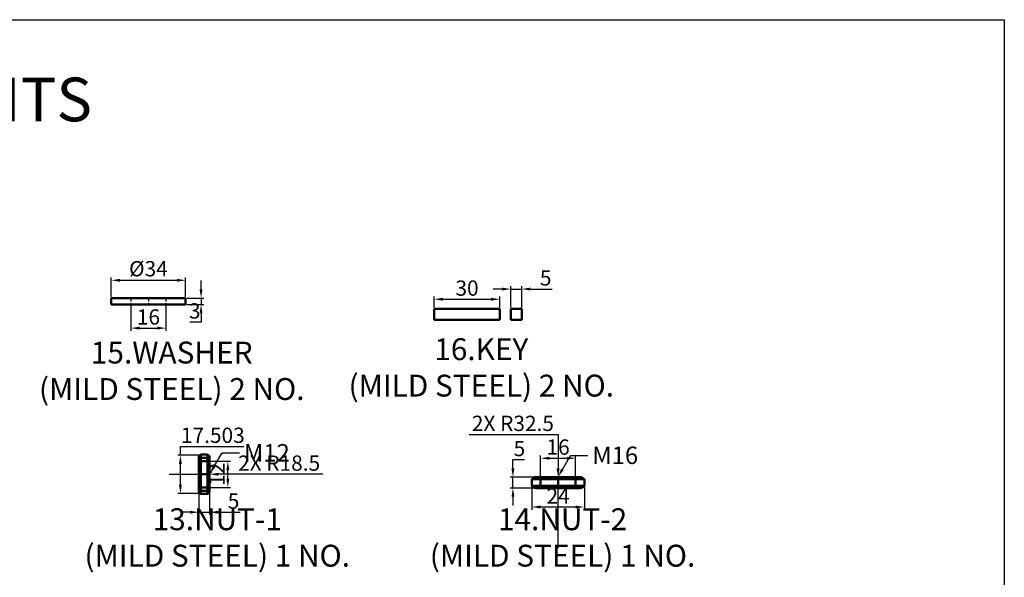
# Model space of a CAD drawing. Units: millimetres. Extents: x -66 to 1195, y -396 to 398.
# Tile 8 of 8: x 745 to 1195, y 143 to 398. Entities that reach past the tile are written whole.
import ezdxf
from ezdxf import colors
from ezdxf.entities.mleader import LeaderData, LeaderLine
from ezdxf.math import Vec2, Vec3

# ---------------------------------------------------------------- set-up
doc = ezdxf.new("R2010")
doc.units = ezdxf.units.MM
doc.header["$LTSCALE"] = 0.5
doc.linetypes.add('HIDDEN', pattern=[9.525, 6.35, -3.175])
for name, color, linetype, lineweight in [('M-DIMS', 2, 'Continuous', 25), ('M-HIDN', 3, 'HIDDEN', 25), ('M-OUTL', 7, 'Continuous', 50), ('M-TEXT', 7, 'Continuous', 25), ('M-TTLB', 7, 'Continuous', 25)]:
    doc.layers.add(name, color=color, linetype=linetype, lineweight=lineweight)
doc.styles.get("Standard").update_dxf_attribs({"font": 'arial.ttf'})
doc.dimstyles.new('ISO-25', dxfattribs={"dimtxt": 7, "dimasz": 4, "dimexe": 1.25, "dimexo": 0.625, "dimtad": 1, "dimtoh": 1, "dimtxsty": 'Standard', "dimcen": 2.5, "dimadec": 0, "dimazin": 0, "dimtfac": 1, "dimtmove": 0, "dimatfit": 3, "dimfxl": 1, "dimarcsym": 0})

# ---------------------------------------------------------------- blocks, each defined once
blk = doc.blocks.new('*D64')
at = {"layer": 'Defpoints', "color": 0, "ltscale": 0.5, "transparency": 16777216}
for p in [(820.76, 278.41), (786.76, 270.29), (820.76, 270.29)]:
    blk.add_point(p, dxfattribs=at)
at = {"layer": 'M-DIMS', "color": 0, "lineweight": -2, "ltscale": 0.5, "transparency": 16777216}
for p, q in [((786.76, 270.91), (786.76, 279.66)), ((820.76, 270.91), (820.76, 279.66)), ((790.76, 278.41), (816.76, 278.41))]:
    blk.add_line(p, q, dxfattribs=at)
at = {"layer": 'M-DIMS', "color": 0, "ltscale": 0.5, "transparency": 16777216}
for points in [[(790.76, 279.08), (790.76, 277.74), (786.76, 278.41)], [(816.76, 279.08), (816.76, 277.74), (820.76, 278.41)]]:
    blk.add_solid(points, dxfattribs=at)
at = {"layer": 'M-DIMS', "color": 0, "ltscale": 0.5, "transparency": 16777216, "insert": (803.76, 282.8), "char_height": 7, "attachment_point": 5}
blk.add_mtext('%%C34', dxfattribs=at)
blk = doc.blocks.new('*D65')
at = {"layer": 'Defpoints', "color": 0, "ltscale": 0.5, "transparency": 16777216}
for p in [(820.76, 270.29), (820.76, 267.29), (827.82, 267.29)]:
    blk.add_point(p, dxfattribs=at)
at = {"layer": 'M-DIMS', "color": 0, "lineweight": -2, "ltscale": 0.5, "transparency": 16777216}
for p, q in [((827.82, 274.29), (827.82, 278.29)), ((821.38, 270.29), (829.07, 270.29)), ((827.82, 270.29), (827.82, 267.29)), ((821.38, 267.29), (829.07, 267.29)), ((827.82, 263.29), (827.82, 259.29)), ((827.82, 259.29), (822.62, 259.29))]:
    blk.add_line(p, q, dxfattribs=at)
at = {"layer": 'M-DIMS', "color": 0, "ltscale": 0.5, "transparency": 16777216}
for points in [[(827.16, 274.29), (828.49, 274.29), (827.82, 270.29)], [(827.16, 263.29), (828.49, 263.29), (827.82, 267.29)]]:
    blk.add_solid(points, dxfattribs=at)
at = {"layer": 'M-DIMS', "color": 0, "ltscale": 0.5, "transparency": 16777216, "insert": (824.91, 263.49), "char_height": 7, "attachment_point": 5}
blk.add_mtext('3', dxfattribs=at)
blk = doc.blocks.new('*D66')
at = {"layer": 'Defpoints', "color": 0, "ltscale": 0.5, "transparency": 16777216}
for p in [(795.76, 267.29), (811.76, 267.29), (811.76, 256.53)]:
    blk.add_point(p, dxfattribs=at)
at = {"layer": 'M-DIMS', "color": 0, "lineweight": -2, "ltscale": 0.5, "transparency": 16777216}
for p, q in [((795.76, 266.66), (795.76, 255.28)), ((811.76, 266.66), (811.76, 255.28)), ((799.76, 256.53), (807.76, 256.53))]:
    blk.add_line(p, q, dxfattribs=at)
at = {"layer": 'M-DIMS', "color": 0, "ltscale": 0.5, "transparency": 16777216}
for points in [[(799.76, 257.2), (799.76, 255.86), (795.76, 256.53)], [(807.76, 257.2), (807.76, 255.86), (811.76, 256.53)]]:
    blk.add_solid(points, dxfattribs=at)
at = {"layer": 'M-DIMS', "color": 0, "ltscale": 0.5, "transparency": 16777216, "insert": (803.76, 260.73), "char_height": 7, "attachment_point": 5}
blk.add_mtext('16', dxfattribs=at)
blk = doc.blocks.new('*D67')
at = {"layer": 'Defpoints', "color": 0, "ltscale": 0.5, "transparency": 16777216}
for p in [(964.42, 269.73), (934.42, 265.35), (964.42, 265.35)]:
    blk.add_point(p, dxfattribs=at)
at = {"layer": 'M-DIMS', "color": 0, "lineweight": -2, "ltscale": 0.5, "transparency": 16777216}
for p, q in [((934.42, 265.97), (934.42, 270.98)), ((964.42, 265.97), (964.42, 270.98)), ((938.42, 269.73), (960.42, 269.73))]:
    blk.add_line(p, q, dxfattribs=at)
at = {"layer": 'M-DIMS', "color": 0, "ltscale": 0.5, "transparency": 16777216}
for points in [[(938.42, 270.4), (938.42, 269.07), (934.42, 269.73)], [(960.42, 270.4), (960.42, 269.07), (964.42, 269.73)]]:
    blk.add_solid(points, dxfattribs=at)
at = {"layer": 'M-DIMS', "color": 0, "ltscale": 0.5, "transparency": 16777216, "insert": (949.42, 273.93), "char_height": 7, "attachment_point": 5}
blk.add_mtext('30', dxfattribs=at)
blk = doc.blocks.new('*D68')
at = {"layer": 'Defpoints', "color": 0, "ltscale": 0.5, "transparency": 16777216}
for p in [(974.42, 274.4), (969.42, 265.35), (974.42, 265.35)]:
    blk.add_point(p, dxfattribs=at)
at = {"layer": 'M-DIMS', "color": 0, "lineweight": -2, "ltscale": 0.5, "transparency": 16777216}
for p, q in [((969.42, 265.97), (969.42, 275.65)), ((974.42, 265.97), (974.42, 275.65)), ((965.42, 274.4), (961.42, 274.4)), ((969.42, 274.4), (974.42, 274.4)), ((978.42, 274.4), (988.31, 274.4))]:
    blk.add_line(p, q, dxfattribs=at)
at = {"layer": 'M-DIMS', "color": 0, "ltscale": 0.5, "transparency": 16777216}
for points in [[(965.42, 275.06), (965.42, 273.73), (969.42, 274.4)], [(978.42, 275.06), (978.42, 273.73), (974.42, 274.4)]]:
    blk.add_solid(points, dxfattribs=at)
at = {"layer": 'M-DIMS', "color": 0, "ltscale": 0.5, "transparency": 16777216, "insert": (985.37, 278.58), "char_height": 7, "attachment_point": 5}
blk.add_mtext('5', dxfattribs=at)
blk = doc.blocks.new('*D109')
at = {"layer": 'Defpoints', "color": 0, "ltscale": 0.5, "transparency": 16777216}
for p in [(818.38, 198.4), (827.32, 198.4), (827.32, 180.9)]:
    blk.add_point(p, dxfattribs=at)
at = {"layer": 'M-DIMS', "color": 0, "lineweight": -2, "ltscale": 0.5, "transparency": 16777216}
for p, q in [((826.7, 198.4), (817.13, 198.4)), ((818.38, 198.4), (818.38, 202.4)), ((818.38, 202.4), (847.41, 202.4)), ((818.38, 184.9), (818.38, 194.4)), ((826.7, 180.9), (817.13, 180.9))]:
    blk.add_line(p, q, dxfattribs=at)
at = {"layer": 'M-DIMS', "color": 0, "ltscale": 0.5, "transparency": 16777216}
for points in [[(817.72, 194.4), (819.05, 194.4), (818.38, 198.4)], [(817.72, 184.9), (819.05, 184.9), (818.38, 180.9)]]:
    blk.add_solid(points, dxfattribs=at)
at = {"layer": 'M-DIMS', "color": 0, "ltscale": 0.5, "transparency": 16777216, "insert": (833.21, 206.6), "char_height": 7, "attachment_point": 5}
blk.add_mtext('17.503', dxfattribs=at)
blk = doc.blocks.new('*D110')
at = {"layer": 'Defpoints', "color": 0, "ltscale": 0.5, "transparency": 16777216}
for p in [(826.73, 189.65), (831.73, 189.65), (831.73, 172.3)]:
    blk.add_point(p, dxfattribs=at)
at = {"layer": 'M-DIMS', "color": 0, "lineweight": -2, "ltscale": 0.5, "transparency": 16777216}
for p, q in [((826.73, 189.02), (826.73, 171.05)), ((831.73, 189.02), (831.73, 171.05)), ((822.73, 172.3), (818.73, 172.3)), ((826.73, 172.3), (831.73, 172.3)), ((835.73, 172.3), (845.63, 172.3))]:
    blk.add_line(p, q, dxfattribs=at)
at = {"layer": 'M-DIMS', "color": 0, "ltscale": 0.5, "transparency": 16777216}
for points in [[(822.73, 172.97), (822.73, 171.63), (826.73, 172.3)], [(835.73, 172.97), (835.73, 171.63), (831.73, 172.3)]]:
    blk.add_solid(points, dxfattribs=at)
at = {"layer": 'M-DIMS', "color": 0, "ltscale": 0.5, "transparency": 16777216, "insert": (842.68, 176.48), "char_height": 7, "attachment_point": 5}
blk.add_mtext('5', dxfattribs=at)
blk = doc.blocks.new('*D111')
at = {"layer": 'Defpoints', "color": 0, "ltscale": 0.5, "transparency": 16777216}
for p in [(831.73, 195.65), (840.08, 195.65), (831.73, 183.65)]:
    blk.add_point(p, dxfattribs=at)
at = {"layer": 'M-DIMS', "color": 0, "lineweight": -2, "ltscale": 0.5, "transparency": 16777216}
for p, q in [((832.36, 195.65), (841.33, 195.65)), ((840.08, 187.65), (840.08, 191.65)), ((832.36, 183.65), (841.33, 183.65))]:
    blk.add_line(p, q, dxfattribs=at)
at = {"layer": 'M-DIMS', "color": 0, "ltscale": 0.5, "transparency": 16777216}
for points in [[(839.42, 191.65), (840.75, 191.65), (840.08, 195.65)], [(839.42, 187.65), (840.75, 187.65), (840.08, 183.65)]]:
    blk.add_solid(points, dxfattribs=at)
at = {"layer": 'M-DIMS', "color": 0, "ltscale": 0.5, "transparency": 16777216, "insert": (835.95, 189.65), "char_height": 7, "attachment_point": 5, "rotation": 90}
blk.add_mtext('12', dxfattribs=at)
blk = doc.blocks.new('*D112')
at = {"layer": 'Defpoints', "color": 0, "ltscale": 0.5, "transparency": 16777216}
for p in [(979.06, 184.34), (1003.06, 184.34), (1003.06, 174.69)]:
    blk.add_point(p, dxfattribs=at)
at = {"layer": 'M-DIMS', "color": 0, "lineweight": -2, "ltscale": 0.5, "transparency": 16777216}
for p, q in [((979.06, 183.72), (979.06, 173.44)), ((1003.06, 183.72), (1003.06, 173.44)), ((983.06, 174.69), (999.06, 174.69))]:
    blk.add_line(p, q, dxfattribs=at)
at = {"layer": 'M-DIMS', "color": 0, "ltscale": 0.5, "transparency": 16777216}
for points in [[(983.06, 175.36), (983.06, 174.02), (979.06, 174.69)], [(999.06, 175.36), (999.06, 174.02), (1003.06, 174.69)]]:
    blk.add_solid(points, dxfattribs=at)
at = {"layer": 'M-DIMS', "color": 0, "ltscale": 0.5, "transparency": 16777216, "insert": (991.06, 178.83), "char_height": 7, "attachment_point": 5}
blk.add_mtext('24', dxfattribs=at)
blk = doc.blocks.new('*D113')
at = {"layer": 'Defpoints', "color": 0, "ltscale": 0.5, "transparency": 16777216}
for p in [(970.41, 188.34), (983.06, 188.34), (983.06, 183.34)]:
    blk.add_point(p, dxfattribs=at)
at = {"layer": 'M-DIMS', "color": 0, "lineweight": -2, "ltscale": 0.5, "transparency": 16777216}
for p, q in [((970.41, 192.34), (970.41, 196.34)), ((970.41, 196.34), (975.68, 196.34)), ((982.44, 188.34), (969.16, 188.34)), ((970.41, 183.34), (970.41, 188.34)), ((982.44, 183.34), (969.16, 183.34)), ((970.41, 179.34), (970.41, 175.34))]:
    blk.add_line(p, q, dxfattribs=at)
at = {"layer": 'M-DIMS', "color": 0, "ltscale": 0.5, "transparency": 16777216}
for points in [[(969.74, 192.34), (971.08, 192.34), (970.41, 188.34)], [(969.74, 179.34), (971.08, 179.34), (970.41, 183.34)]]:
    blk.add_solid(points, dxfattribs=at)
at = {"layer": 'M-DIMS', "color": 0, "ltscale": 0.5, "transparency": 16777216, "insert": (973.36, 200.53), "char_height": 7, "attachment_point": 5}
blk.add_mtext('5', dxfattribs=at)
blk = doc.blocks.new('*D114')
at = {"layer": 'Defpoints', "color": 0, "ltscale": 0.5, "transparency": 16777216}
for p in [(999.06, 197), (983.06, 188.34), (999.06, 188.34)]:
    blk.add_point(p, dxfattribs=at)
at = {"layer": 'M-DIMS', "color": 0, "lineweight": -2, "ltscale": 0.5, "transparency": 16777216}
for p, q in [((983.06, 188.97), (983.06, 198.25)), ((999.06, 188.97), (999.06, 198.25)), ((987.06, 197), (995.06, 197))]:
    blk.add_line(p, q, dxfattribs=at)
at = {"layer": 'M-DIMS', "color": 0, "ltscale": 0.5, "transparency": 16777216}
for points in [[(987.06, 197.66), (987.06, 196.33), (983.06, 197)], [(995.06, 197.66), (995.06, 196.33), (999.06, 197)]]:
    blk.add_solid(points, dxfattribs=at)
at = {"layer": 'M-DIMS', "color": 0, "ltscale": 0.5, "transparency": 16777216, "insert": (991.06, 201.2), "char_height": 7, "attachment_point": 5}
blk.add_mtext('16', dxfattribs=at)
blk = doc.blocks.new('*D133')
at = {"layer": 'Defpoints', "color": 0, "ltscale": 0.5, "transparency": 16777216}
for p in [(813.23, 189.65), (831.73, 189.65)]:
    blk.add_point(p, dxfattribs=at)
at = {"layer": 'M-DIMS', "color": 0, "lineweight": -2, "ltscale": 0.5, "transparency": 16777216}
for p, q in [((813.23, 189.65), (831.73, 189.65)), ((842.83, 189.65), (835.73, 189.65)), ((883.55, 189.65), (842.83, 189.65))]:
    blk.add_line(p, q, dxfattribs=at)
at = {"layer": 'M-DIMS', "color": 0, "ltscale": 0.5, "transparency": 16777216}
blk.add_solid([(835.73, 190.32), (835.73, 188.98), (831.73, 189.65)], dxfattribs=at)
at = {"layer": 'M-DIMS', "color": 0, "ltscale": 0.5, "transparency": 16777216, "insert": (863.51, 193.85), "char_height": 7, "attachment_point": 5}
blk.add_mtext('2X R18.5', dxfattribs=at)
blk = doc.blocks.new('*D134')
at = {"layer": 'Defpoints', "color": 0, "ltscale": 0.5, "transparency": 16777216}
for p in [(991.06, 188.34), (991.06, 155.84)]:
    blk.add_point(p, dxfattribs=at)
at = {"layer": 'M-DIMS', "color": 0, "lineweight": -2, "ltscale": 0.5, "transparency": 16777216}
for p, q in [((950.34, 207.84), (991.06, 207.84)), ((991.06, 207.84), (991.06, 192.34)), ((991.06, 155.84), (991.06, 188.34))]:
    blk.add_line(p, q, dxfattribs=at)
at = {"layer": 'M-DIMS', "color": 0, "ltscale": 0.5, "transparency": 16777216}
blk.add_solid([(991.73, 192.34), (990.39, 192.34), (991.06, 188.34)], dxfattribs=at)
at = {"layer": 'M-DIMS', "color": 0, "ltscale": 0.5, "transparency": 16777216, "insert": (970.39, 212.05), "char_height": 7, "attachment_point": 5}
blk.add_mtext('2X R32.5', dxfattribs=at)

msp = doc.modelspace()

# ---------------------------------------------------------------- linework, layer by layer
at = {"layer": 'M-HIDN', "ltscale": 0.5}
for p, q in [((795.7565, 270.2874), (795.7565, 267.2874)), ((803.7565, 270.2874), (803.7565, 267.2874)), ((811.7565, 270.2874), (811.7565, 267.2874))]:
    msp.add_line(p, q, dxfattribs=at)
at = {"layer": 'M-OUTL', "ltscale": 0.5}
for p, q in [((786.7565, 270.2874), (820.7565, 270.2874)), ((786.7565, 267.2874), (786.7565, 270.2874)), ((820.7565, 270.2874), (820.7565, 267.2874)), ((820.7565, 267.2874), (786.7565, 267.2874)), ((934.4214, 265.3451), (964.4214, 265.3451)), ((934.4214, 260.3451), (934.4214, 265.3451)), ((964.4214, 265.3451), (964.4214, 260.3451)), ((969.4214, 265.3451), (974.4214, 265.3451)), ((969.4214, 260.3451), (969.4214, 265.3451)), ((974.4214, 265.3451), (974.4214, 260.3451)), ((964.4214, 260.3451), (934.4214, 260.3451)), ((974.4214, 260.3451), (969.4214, 260.3451)), ((830.7347, 198.6487), (827.7347, 198.6487)), ((827.7347, 180.6487), (827.7347, 198.6487)), ((830.7347, 180.6487), (830.7347, 198.6487)), ((826.7347, 197.1487), (826.7347, 182.1487)), ((831.7347, 197.1487), (826.7347, 197.1487)), ((826.7347, 182.1487), (826.7347, 197.1487)), ((826.7347, 195.6487), (831.7347, 195.6487)), ((831.7347, 182.1487), (831.7347, 197.1487)), ((826.7347, 189.6487), (831.7347, 189.6487)), ((979.0602, 187.3437), (979.0602, 184.3437)), ((979.0602, 187.3437), (1003.0602, 187.3437)), ((980.9441, 188.3437), (1001.0707, 188.3437)), ((983.0602, 183.3437), (983.0602, 188.3437)), ((991.0602, 188.3437), (991.0602, 183.3437)), ((999.0602, 188.3437), (999.0602, 183.3437)), ((1003.0602, 187.3437), (1003.0602, 184.3437)), ((826.7347, 183.6487), (831.7347, 183.6487)), ((826.7347, 182.1487), (831.7347, 182.1487)), ((827.7347, 180.6487), (830.7347, 180.6487)), ((979.0602, 184.3437), (1003.0602, 184.3437)), ((980.9441, 183.3437), (983.0602, 183.3437)), ((980.9441, 183.3437), (1001.0707, 183.3437)), ((999.0602, 183.3437), (983.0602, 183.3437)), ((1001.0707, 183.3437), (999.0602, 183.3437))]:
    msp.add_line(p, q, dxfattribs=at)
for centre, radius, start, end in [((828.3597, 197.1487), 1.625, 112.619865, 247.380135), ((830.1097, 197.1487), 1.625, 292.619865, 67.380135), ((845.2347, 189.6487), 18.5, 161.075356, 198.924644), ((813.2347, 189.6487), 18.5, 341.075356, 18.924644), ((981.0602, 185.8505), 2.496, 36.745976, 143.254024), ((991.0602, 155.8437), 32.5, 75.749967, 104.250033), ((1001.0602, 185.8438), 2.5, 36.868896, 143.131104), ((828.3597, 182.1487), 1.625, 112.619865, 247.380135), ((830.1097, 182.1487), 1.625, 292.619865, 67.380135), ((981.0602, 185.837), 2.496, 216.745976, 323.254024), ((991.0602, 215.8437), 32.5, 255.749967, 284.250033), ((1001.0602, 185.8437), 2.5, 216.868896, 323.131104)]:
    msp.add_arc(centre, radius, start, end, dxfattribs=at)
at = {"layer": 'M-TTLB', "ltscale": 0.5}
msp.add_lwpolyline([(-66.4176, 397.641), (1195.0519, 397.641), (1195.0519, -395.6964), (-66.4176, -395.6964)], close=True, dxfattribs=at)

# ---------------------------------------------------------------- texts
at = {"layer": 'M-TEXT', "ltscale": 0.5, "attachment_point": 1}
for s, width, insert, char_height in [('LATHE TAIL STOCK COMPONENTS ', 485.790741, (346.8576, 371.1482), 20), ('\\pxqc;15.WASHER \\P(MILD STEEL) 2 NO.', 203.992441, (712.4274, 250.3326), 10), ('\\pxqc;16.KEY \\P(MILD STEEL) 2 NO.', 203.992441, (853.9471, 251.883), 10), ('\\pxqc;13.NUT-1\\P(MILD STEEL) 1 NO.', 203.992441, (733.2302, 174.0776), 10), ('\\pxqc;14.NUT-2\\P(MILD STEEL) 1 NO.', 203.992441, (891.0952, 174.0776), 10)]:
    msp.add_mtext_dynamic_manual_height_columns(s, width=width, gutter_width=12.5, heights=[0], dxfattribs=dict(at, insert=insert, char_height=char_height))

# ---------------------------------------------------------------- dimensions: what is measured, and where the dimension line sits
at = {"layer": 'M-DIMS', "ltscale": 0.5}
dim = msp.add_linear_dim(base=(820.7565, 278.4092), p1=(786.7565, 270.2874), p2=(820.7565, 270.2874), text='%%C<>', dimstyle='ISO-25', override={"dimclrd": 0, "dimclre": 0, "dimclrt": 0}, dxfattribs=at)
dim.commit()
dim.dimension.update_dxf_attribs({"geometry": '*D64', "text_midpoint": (803.7565, 282.8039)})
for base, p1, p2, override, picture, middle in [((974.4214, 274.3973), (969.4214, 265.3451), (974.4214, 265.3451), {"dimclrd": 0, "dimclre": 0, "dimclrt": 0}, '*D68', (985.367, 278.5819)), ((964.4214, 269.7327), (934.4214, 265.3451), (964.4214, 265.3451), {"dimclrd": 0, "dimclre": 0, "dimclrt": 0}, '*D67', (949.4214, 273.9341)), ((811.7565, 256.5312), (795.7565, 267.2874), (811.7565, 267.2874), {"dimclrd": 0, "dimclre": 0, "dimclrt": 0}, '*D66', (803.7565, 260.7302)), ((999.0602, 196.9964), (983.0602, 188.3437), (999.0602, 188.3437), {"dimdec": 0, "dimlfac": 1, "dimrnd": 0, "dimzin": 0, "dimdsep": 46, "dimlunit": 2}, '*D114', (991.0602, 201.1954)), ((831.7347, 172.2987), (826.7347, 189.6487), (831.7347, 189.6487), {"dimdec": 0, "dimlfac": 1, "dimrnd": 0, "dimzin": 0, "dimdsep": 46, "dimlunit": 2}, '*D110', (842.6803, 176.4834)), ((1003.0602, 174.691), (979.0602, 184.3437), (1003.0602, 184.3437), {"dimdec": 0, "dimlfac": 1, "dimrnd": 0, "dimzin": 0, "dimdsep": 46, "dimlunit": 2}, '*D112', (991.0602, 178.8303))]:
    dim = msp.add_linear_dim(base=base, p1=p1, p2=p2, dimstyle='ISO-25', override=override, dxfattribs=at)
    dim.commit()
    dim.dimension.update_dxf_attribs({"geometry": picture, "text_midpoint": middle})
for base, p1, p2, override, picture, middle in [((827.824, 267.2874), (820.7565, 270.2874), (820.7565, 267.2874), {"dimclrd": 0, "dimclre": 0, "dimclrt": 0}, '*D65', (824.9071, 263.4888)), ((818.3847, 198.4001), (827.323, 180.8972), (827.323, 198.4001), {"dimdec": 3, "dimlfac": 1, "dimrnd": 0, "dimzin": 0, "dimdsep": 46, "dimlunit": 2}, '*D109', (833.2103, 206.6015)), ((970.4102, 188.3437), (983.0602, 183.3437), (983.0602, 188.3437), {"dimdec": 0, "dimlfac": 1, "dimrnd": 0, "dimzin": 0, "dimdsep": 46, "dimlunit": 2}, '*D113', (973.3558, 200.5284)), ((840.0847, 195.6487), (831.7347, 183.6487), (831.7347, 195.6487), {"dimdec": 0, "dimlfac": 1, "dimrnd": 0, "dimzin": 0, "dimdsep": 46, "dimlunit": 2}, '*D111', (835.9454, 189.6487))]:
    dim = msp.add_linear_dim(base=base, p1=p1, p2=p2, angle=90, dimstyle='ISO-25', override=override, dxfattribs=at)
    dim.commit()
    dim.dimension.update_dxf_attribs({"geometry": picture, "text_midpoint": middle})
for center, mpoint, picture, middle in [((991.0602, 155.8437), (991.06, 188.3437), '*D134', (970.3874, 207.8437)), ((813.2347, 189.6487), (831.7347, 189.65), '*D133', (842.8347, 189.6508))]:
    dim = msp.add_radius_dim(center=center, mpoint=mpoint, text='2X <>', dimstyle='ISO-25', override={"dimdec": 1, "dimlfac": 1, "dimrnd": 0, "dimzin": 0, "dimdsep": 46, "dimlunit": 2}, dxfattribs=at)
    dim.commit()
    dim.dimension.update_dxf_attribs({"geometry": picture, "text_midpoint": middle, "dimtype": 164})

# ---------------------------------------------------------------- leaders
at = {"layer": 'M-TEXT', "ltscale": 0.5}
ml = msp.add_multileader_mtext('Standard', dxfattribs=at)
ml.set_content('M12', color=256)
ml.set_leader_properties()
ml.build(insert=Vec2(0, 0))
ctx = ml.context
ctx.base_point, ctx.char_height, ctx.plane_origin = Vec3(845.4087, 199.4763), 8, Vec3(831.7347, 189.6487)
notes = []
notes.append((ctx, [(0, (1, 1, 0), (837.4087, 199.4763), (1, 0), 8, [(0, [(831.7347, 189.6487)], 0, [])])]))
ctx.mtext.insert, ctx.mtext.flow_direction = Vec3(847.4087, 203.4763), 5
ml = msp.add_multileader_mtext('Standard', dxfattribs=at)
ml.set_content('M16', color=256)
ml.set_leader_properties()
ml.build(insert=Vec2(0, 0))
ctx = ml.context
ctx.base_point, ctx.char_height, ctx.plane_origin = Vec3(1004.6814, 198.2629), 8, Vec3(991.0074, 188.4353)
notes.append((ctx, [(0, (1, 1, 0), (996.6814, 198.2629), (1, 0), 8, [(0, [(991.0074, 188.4353)], 0, [])])]))
ctx.mtext.insert, ctx.mtext.flow_direction = Vec3(1006.6814, 202.3311), 5
for ctx, leaders in notes:
    for number, flags, end, landing, length, lines in leaders:
        leader = LeaderData()
        leader.index, (leader.has_last_leader_line, leader.has_dogleg_vector, leader.attachment_direction) = number, flags
        leader.last_leader_point, leader.dogleg_vector, leader.dogleg_length = Vec3(end), Vec3(landing), length
        for number, points, colour, breaks in lines:
            line = LeaderLine()
            line.index, line.vertices, line.color, line.breaks = number, Vec3.list(points), colors.encode_raw_color(colour), breaks
            leader.lines.append(line)
        ctx.leaders.append(leader)

doc.saveas('drawing.dxf')
